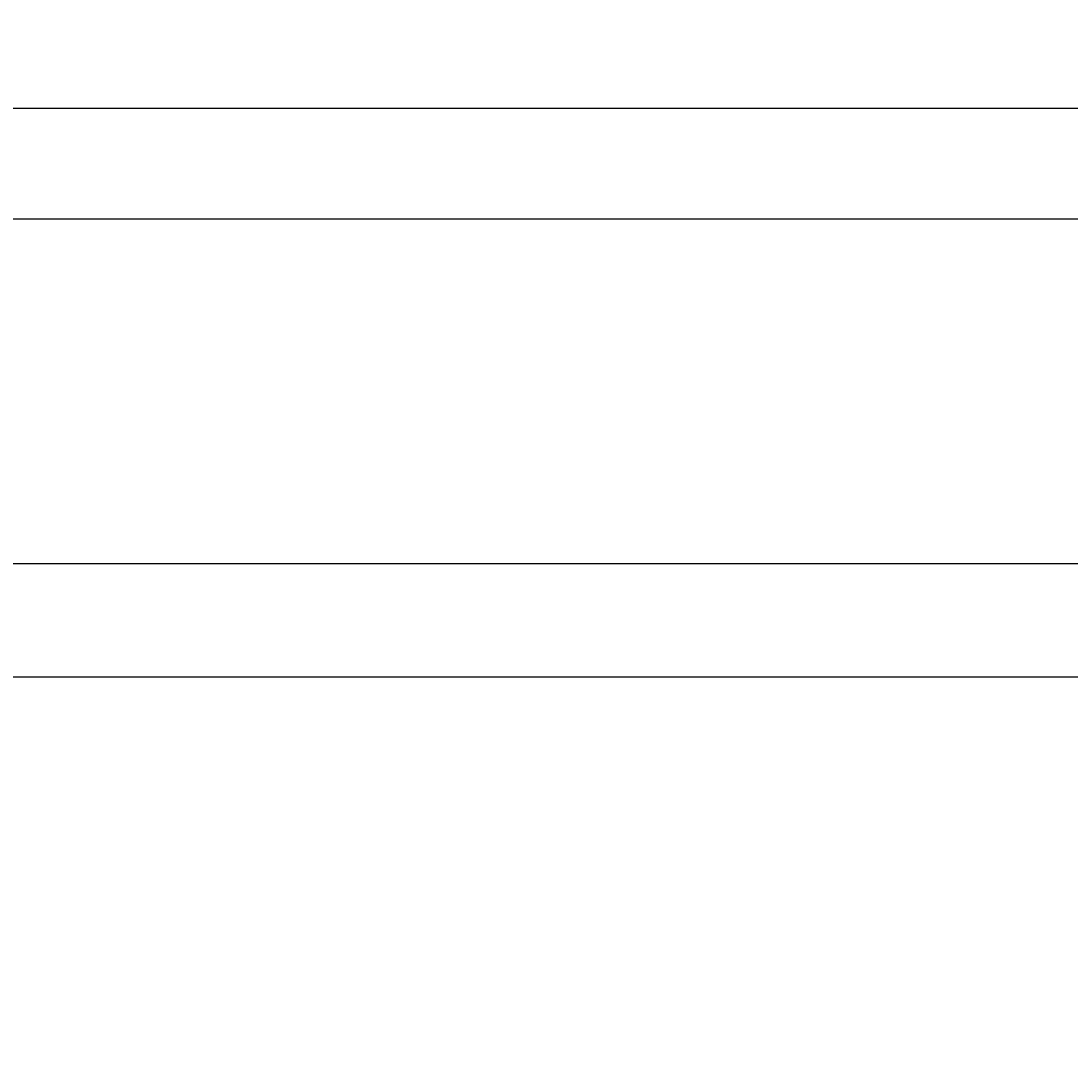
# Model space of a CAD drawing. Units: inches. Extents: x 35362 to 73946, y 43607 to 67532.
# Tile 62 of 134: x 48533 to 49302, y 46919 to 47689. Entities that reach past the tile are written whole.
import ezdxf

# ---------------------------------------------------------------- set-up
doc = ezdxf.new("R2010")
doc.units = ezdxf.units.IN
doc.header["$MEASUREMENT"] = 0
doc.layers.add('A-ANNO-DIMS', color=2, linetype='Continuous', lineweight=18)
doc.styles.get("Standard").update_dxf_attribs({"font": 'arial.ttf'})
doc.dimstyles.get("Standard").update_dxf_attribs({"dimtxt": 0.18, "dimasz": 0.18, "dimexe": 0.18, "dimexo": 0.0625, "dimgap": 0.09, "dimtad": 0, "dimtih": 1, "dimtoh": 1, "dimdec": 4, "dimzin": 0, "dimdsep": 46, "dimtxsty": 'Standard', "dimcen": 0.09, "dimadec": 0, "dimazin": 0, "dimtfac": 1, "dimtdec": 4, "dimtofl": 0, "dimtmove": 0, "dimatfit": 3, "dimfxl": 1, "dimtolj": 1, "dimtzin": 0, "dimarcsym": 0})

# ---------------------------------------------------------------- blocks, each defined once
blk = doc.blocks.new('*D11')
at = {"layer": 'A-ANNO-DIMS', "color": 0, "lineweight": -2, "transparency": 16777216}
for p, q in [((47978.66, 56028.77), (47978.66, 43606.68)), ((53109.76, 56028.77), (53109.76, 43606.68)), ((47978.84, 43606.86), (50543.87, 43606.86)), ((53109.58, 43606.86), (50544.55, 43606.86))]:
    blk.add_line(p, q, dxfattribs=at)
at = {"layer": 'A-ANNO-DIMS', "color": 0, "transparency": 16777216}
for points in [[(47978.84, 43606.89), (47978.84, 43606.83), (47978.66, 43606.86)], [(53109.58, 43606.89), (53109.58, 43606.83), (53109.76, 43606.86)]]:
    blk.add_solid(points, dxfattribs=at)
at = {"layer": 'Defpoints', "color": 0, "transparency": 16777216}
for p in [(47978.66, 56028.84), (53109.76, 56028.84), (53109.76, 43606.86)]:
    blk.add_point(p, dxfattribs=at)
at = {"layer": 'A-ANNO-DIMS', "color": 0, "transparency": 16777216, "insert": (50544.21, 43606.86), "char_height": 0.18, "attachment_point": 5}
blk.add_mtext('\\A1;5131', dxfattribs=at)
blk = doc.blocks.new('*D13')
at = {"layer": 'A-ANNO-DIMS', "color": 0, "lineweight": -2, "transparency": 16777216}
for p, q in [((48373.49, 51694.02), (48373.49, 43606.68)), ((51029.04, 51694.02), (51029.04, 43606.68)), ((48373.67, 43606.86), (49700.8, 43606.86)), ((51028.86, 43606.86), (49701.73, 43606.86))]:
    blk.add_line(p, q, dxfattribs=at)
at = {"layer": 'A-ANNO-DIMS', "color": 0, "transparency": 16777216}
for points in [[(48373.67, 43606.89), (48373.67, 43606.83), (48373.49, 43606.86)], [(51028.86, 43606.89), (51028.86, 43606.83), (51029.04, 43606.86)]]:
    blk.add_solid(points, dxfattribs=at)
at = {"layer": 'Defpoints', "color": 0, "transparency": 16777216}
for p in [(48373.49, 51694.09), (51029.04, 51694.09), (51029.04, 43606.86)]:
    blk.add_point(p, dxfattribs=at)
at = {"layer": 'A-ANNO-DIMS', "color": 0, "transparency": 16777216, "insert": (49701.27, 43606.86), "char_height": 0.18, "attachment_point": 5}
blk.add_mtext('\\A1;2655.6', dxfattribs=at)
blk = doc.blocks.new('*D43')
at = {"layer": 'A-ANNO-DIMS', "color": 0, "lineweight": -2, "transparency": 16777216}
for p, q in [((62004.67, 47625.18), (35361.77, 47625.18)), ((35361.95, 47625), (35361.95, 47416.9)), ((35361.95, 47208.43), (35361.95, 47416.53)), ((62004.67, 47208.25), (35361.77, 47208.25))]:
    blk.add_line(p, q, dxfattribs=at)
at = {"layer": 'A-ANNO-DIMS', "color": 0, "transparency": 16777216}
for points in [[(35361.92, 47625), (35361.98, 47625), (35361.95, 47625.18)], [(35361.92, 47208.43), (35361.98, 47208.43), (35361.95, 47208.25)]]:
    blk.add_solid(points, dxfattribs=at)
at = {"layer": 'Defpoints', "color": 0, "transparency": 16777216}
for p in [(62004.73, 47625.18), (35361.95, 47208.25), (62004.73, 47208.25)]:
    blk.add_point(p, dxfattribs=at)
at = {"layer": 'A-ANNO-DIMS', "color": 0, "transparency": 16777216, "insert": (35361.95, 47416.72), "char_height": 0.18, "attachment_point": 5}
blk.add_mtext('\\A1;416.9', dxfattribs=at)
blk = doc.blocks.new('*D67')
at = {"layer": 'A-ANNO-DIMS', "color": 0, "lineweight": -2, "transparency": 16777216}
for p, q in [((56873.54, 53351.53), (35361.77, 53351.53)), ((35361.95, 53351.35), (35361.95, 49400.89)), ((35361.95, 45450.07), (35361.95, 49400.53)), ((53793.58, 45449.89), (35361.77, 45449.89))]:
    blk.add_line(p, q, dxfattribs=at)
at = {"layer": 'A-ANNO-DIMS', "color": 0, "transparency": 16777216}
for points in [[(35361.92, 53351.35), (35361.98, 53351.35), (35361.95, 53351.53)], [(35361.92, 45450.07), (35361.98, 45450.07), (35361.95, 45449.89)]]:
    blk.add_solid(points, dxfattribs=at)
at = {"layer": 'Defpoints', "color": 0, "transparency": 16777216}
for p in [(35361.95, 53351.53), (56873.6, 53351.53), (53793.64, 45449.89)]:
    blk.add_point(p, dxfattribs=at)
at = {"layer": 'A-ANNO-DIMS', "color": 0, "transparency": 16777216, "insert": (35361.95, 49400.71), "char_height": 0.18, "attachment_point": 5}
blk.add_mtext('\\A1;7901.6', dxfattribs=at)
blk = doc.blocks.new('*D87')
at = {"layer": 'A-ANNO-DIMS', "color": 0, "lineweight": -2, "transparency": 16777216}
for p, q in [((52362.49, 48318.27), (35361.77, 48318.27)), ((35361.95, 48318.09), (35361.95, 47931.38)), ((35361.95, 47544.31), (35361.95, 47931.02)), ((52362.49, 47544.13), (35361.77, 47544.13))]:
    blk.add_line(p, q, dxfattribs=at)
at = {"layer": 'A-ANNO-DIMS', "color": 0, "transparency": 16777216}
for points in [[(35361.92, 48318.09), (35361.98, 48318.09), (35361.95, 48318.27)], [(35361.92, 47544.31), (35361.98, 47544.31), (35361.95, 47544.13)]]:
    blk.add_solid(points, dxfattribs=at)
at = {"layer": 'Defpoints', "color": 0, "transparency": 16777216}
for p in [(35361.95, 48318.27), (52362.56, 48318.27), (52362.56, 47544.13)]:
    blk.add_point(p, dxfattribs=at)
at = {"layer": 'A-ANNO-DIMS', "color": 0, "transparency": 16777216, "insert": (35361.95, 47931.2), "char_height": 0.18, "attachment_point": 5}
blk.add_mtext('\\A1;774.1', dxfattribs=at)
blk = doc.blocks.new('*D90')
at = {"layer": 'A-ANNO-DIMS', "color": 0, "lineweight": -2, "transparency": 16777216}
for p, q in [((53707.72, 47291.29), (35361.77, 47291.29)), ((35361.95, 47291.11), (35361.95, 46710.26)), ((35361.95, 46129.06), (35361.95, 46709.9)), ((53793.58, 46128.88), (35361.77, 46128.88))]:
    blk.add_line(p, q, dxfattribs=at)
at = {"layer": 'A-ANNO-DIMS', "color": 0, "transparency": 16777216}
for points in [[(35361.92, 47291.11), (35361.98, 47291.11), (35361.95, 47291.29)], [(35361.92, 46129.06), (35361.98, 46129.06), (35361.95, 46128.88)]]:
    blk.add_solid(points, dxfattribs=at)
at = {"layer": 'Defpoints', "color": 0, "transparency": 16777216}
for p in [(53707.78, 47291.29), (35361.95, 46128.88), (53793.64, 46128.88)]:
    blk.add_point(p, dxfattribs=at)
at = {"layer": 'A-ANNO-DIMS', "color": 0, "transparency": 16777216, "insert": (35361.95, 46710.08), "char_height": 0.18, "attachment_point": 5}
blk.add_mtext('\\A1;1162.4', dxfattribs=at)

msp = doc.modelspace()

# ---------------------------------------------------------------- dimensions: what is measured, and where the dimension line sits
at = {"layer": 'A-ANNO-DIMS'}
for base, p1, p2, override, picture, middle in [((53109.76, 43606.859), (47978.665, 56028.836), (53109.76, 56028.836), {"dimdec": 0, "dimlfac": 1, "dimrnd": 0, "dimzin": 0, "dimdsep": 46, "dimlunit": 2}, '*D11', (50544.212, 43606.859)), ((51029.043, 43606.859), (48373.492, 51694.087), (51029.043, 51694.087), {"dimdec": 1, "dimlfac": 1, "dimrnd": 0, "dimzin": 0, "dimdsep": 46, "dimlunit": 2}, '*D13', (49701.267, 43606.859))]:
    dim = msp.add_linear_dim(base=base, p1=p1, p2=p2, dimstyle='Standard', override=override, dxfattribs=at)
    dim.commit()
    dim.dimension.update_dxf_attribs({"geometry": picture, "text_midpoint": middle})
for base, p1, p2, picture, middle in [((35361.949, 53351.529), (53793.638, 45449.894), (56873.602, 53351.529), '*D67', (35361.949, 49400.712)), ((35361.949, 48318.269), (52362.557, 47544.134), (52362.557, 48318.269), '*D87', (35361.949, 47931.201)), ((35361.949, 47208.25), (62004.728, 47625.181), (62004.728, 47208.25), '*D43', (35361.949, 47416.715)), ((35361.949, 46128.878), (53707.781, 47291.285), (53793.638, 46128.878), '*D90', (35361.949, 46710.081))]:
    dim = msp.add_linear_dim(base=base, p1=p1, p2=p2, angle=90, dimstyle='Standard', override={"dimdec": 1, "dimlfac": 1, "dimrnd": 0, "dimzin": 0, "dimdsep": 46, "dimlunit": 2}, dxfattribs=at)
    dim.commit()
    dim.dimension.update_dxf_attribs({"geometry": picture, "text_midpoint": middle})

doc.saveas('drawing.dxf')
